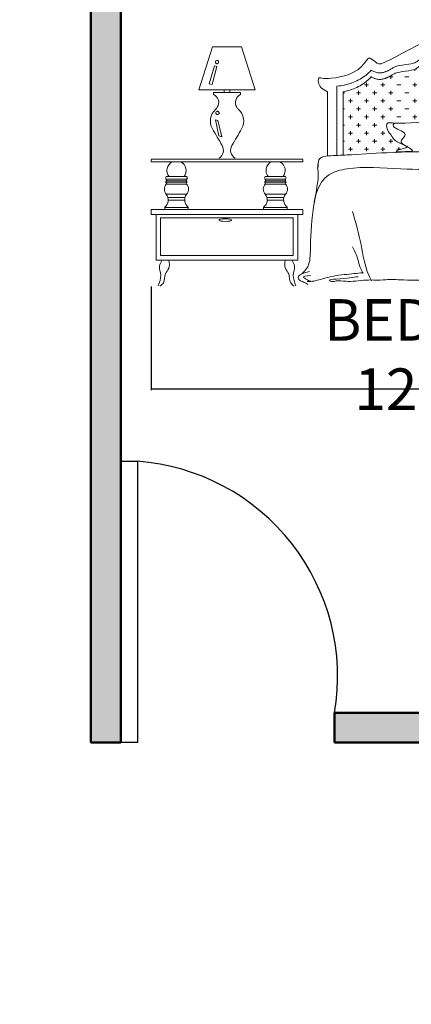
# Model space of a CAD drawing. Units: inches. Extents: x 1771 to 3025, y 319 to 889.
# Tile 20 of 35: x 2390 to 2456, y 621 to 786. Entities that reach past the tile are written whole.
import ezdxf

# ---------------------------------------------------------------- set-up
doc = ezdxf.new("R2010")
doc.units = ezdxf.units.IN
doc.header["$MEASUREMENT"] = 0
for name, color, linetype, lineweight in [('A-ANNO-DIMS', 2, 'Continuous', 18), ('A-AREA-IDEN', 241, 'Continuous', 25), ('A-DOOR', 4, 'Continuous', 25), ('A-FURN', 8, 'Continuous', 18), ('A-WALL', 7, 'Continuous', 50), ('A-WALL-PATT', 254, 'Continuous', 13)]:
    doc.layers.add(name, color=color, linetype=linetype, lineweight=lineweight)
doc.styles.get("Standard").update_dxf_attribs({"font": 'arial.ttf'})
doc.dimstyles.get("Standard").update_dxf_attribs({"dimtxt": 0.18, "dimasz": 0.18, "dimexe": 0.18, "dimexo": 0.0625, "dimgap": 0.09, "dimtad": 0, "dimtih": 1, "dimtoh": 1, "dimdec": 4, "dimzin": 0, "dimdsep": 46, "dimtxsty": 'Standard', "dimcen": 0.09, "dimadec": 0, "dimazin": 0, "dimtfac": 1, "dimtdec": 4, "dimtofl": 0, "dimtmove": 0, "dimatfit": 3, "dimfxl": 1, "dimtolj": 1, "dimtzin": 0, "dimarcsym": 0})

# ---------------------------------------------------------------- blocks, each defined once
blk = doc.blocks.new('A$C3F6F0378')
for p, q in [((188.6, 774.2), (242.7, 943.6)), ((356.2, 943.6), (242.7, 943.6)), ((410.4, 774.2), (356.2, 943.6)), ((1198.7, 944.7), (1198.7, 946.2)), ((1254.2, 952.6), (1270.1, 952.6)), ((1262.2, 944.7), (1262.2, 960.5)), ((1317.7, 952.6), (1333.6, 952.6)), ((1325.7, 944.7), (1325.7, 960.5)), ((1381.2, 952.6), (1397.1, 952.6)), ((1389.2, 944.7), (1389.2, 959.9)), ((2294.6, 774.2), (2348.7, 943.6)), ((2462.2, 943.6), (2348.7, 943.6)), ((2516.4, 774.2), (2462.2, 943.6)), ((1135.2, 881.2), (1135.2, 897)), ((1162.7, 920.9), (1174.9, 920.9)), ((1166.9, 912.9), (1166.9, 924)), ((1198.7, 881.2), (1198.7, 897)), ((1222.5, 920.9), (1238.4, 920.9)), ((1230.4, 912.9), (1230.4, 928.8)), ((1262.2, 881.2), (1262.2, 897)), ((1286, 920.9), (1301.9, 920.9)), ((1293.9, 912.9), (1293.9, 928.8)), ((1325.7, 881.2), (1325.7, 897)), ((1349.5, 920.9), (1365.4, 920.9)), ((1357.4, 912.9), (1357.4, 928.8)), ((1389.2, 881.2), (1389.2, 897)), ((1413, 920.9), (1428.9, 920.9)), ((1420.9, 912.9), (1420.9, 928.8)), ((1452.7, 881.2), (1452.7, 897)), ((1476.5, 920.9), (1485.8, 920.9)), ((1484.4, 912.9), (1484.4, 921.6)), ((1516.2, 881.2), (1516.2, 897)), ((1579.7, 881.2), (1579.7, 897)), ((229, 797.8), (250.3, 869.3)), ((259.4, 866.2), (241.2, 794.8)), ((250.3, 869.3), (259.4, 866.2)), ((1039.9, 849.4), (1039.9, 855.2)), ((1044.6, 857.4), (1047.9, 857.4)), ((1095.5, 857.4), (1111.4, 857.4)), ((1103.4, 849.4), (1103.4, 865.3)), ((1127.2, 889.1), (1143.1, 889.1)), ((1159, 857.4), (1174.9, 857.4)), ((1166.9, 849.4), (1166.9, 865.3)), ((1190.7, 889.1), (1206.6, 889.1)), ((1222.5, 857.4), (1238.4, 857.4)), ((1230.4, 849.4), (1230.4, 865.3)), ((1254.2, 889.1), (1270.1, 889.1)), ((1286, 857.4), (1301.9, 857.4)), ((1293.9, 849.4), (1293.9, 865.3)), ((1317.7, 889.1), (1333.6, 889.1)), ((1349.5, 857.4), (1365.4, 857.4)), ((1357.4, 849.4), (1357.4, 865.3)), ((1381.2, 889.1), (1397.1, 889.1)), ((1413, 857.4), (1428.9, 857.4)), ((1420.9, 849.4), (1420.9, 865.3)), ((1444.7, 889.1), (1460.6, 889.1)), ((1476.5, 857.4), (1492.4, 857.4)), ((1484.4, 849.4), (1484.4, 865.3)), ((1508.2, 889.1), (1524.1, 889.1)), ((1540, 857.4), (1555.9, 857.4)), ((1547.9, 849.4), (1547.9, 865.3)), ((1571.7, 889.1), (1587.6, 889.1)), ((1603.5, 857.4), (1619.4, 857.4)), ((1611.4, 849.4), (1611.4, 865.3)), ((2335.1, 797.8), (2356.3, 869.3)), ((2365.5, 866.2), (2347.3, 794.8)), ((2356.3, 869.3), (2365.5, 866.2)), ((881.2, 817.7), (881.2, 818.8)), ((937.5, 825.6), (952.6, 825.6)), ((944.7, 817.7), (944.7, 829.4)), ((1000.2, 825.6), (1016.1, 825.6)), ((1063.7, 825.6), (1079.6, 825.6)), ((1071.7, 817.7), (1071.7, 833.5)), ((1127.2, 825.6), (1143.1, 825.6)), ((1135.2, 817.7), (1135.2, 833.5)), ((1190.7, 825.6), (1206.6, 825.6)), ((1198.7, 817.7), (1198.7, 833.5)), ((1254.2, 825.6), (1270.1, 825.6)), ((1262.2, 817.7), (1262.2, 833.5)), ((1317.7, 825.6), (1333.6, 825.6)), ((1325.7, 817.7), (1325.7, 833.5)), ((1381.2, 825.6), (1397.1, 825.6)), ((1389.2, 817.7), (1389.2, 833.5)), ((1444.7, 825.6), (1460.6, 825.6)), ((1452.7, 817.7), (1452.7, 833.5)), ((1508.2, 825.6), (1524.1, 825.6)), ((1516.2, 817.7), (1516.2, 833.5)), ((1571.7, 825.6), (1587.6, 825.6)), ((1579.7, 817.7), (1579.7, 833.5)), ((1635.2, 825.6), (1651.1, 825.6)), ((1643.2, 817.7), (1643.2, 833.5)), ((1698.7, 825.6), (1714.6, 825.6)), ((1706.7, 817.7), (1706.7, 828.2)), ((1770.2, 818.9), (1770.2, 818.9)), ((241.2, 794.8), (229, 797.8)), ((841.5, 793.9), (857.4, 793.9)), ((849.4, 785.9), (849.4, 801.8)), ((905, 793.9), (920.9, 793.9)), ((912.9, 785.9), (912.9, 801.8)), ((968.5, 793.9), (984.4, 793.9)), ((1032, 793.9), (1047.9, 793.9)), ((1039.9, 785.9), (1039.9, 801.8)), ((1095.5, 793.9), (1111.4, 793.9)), ((1103.4, 785.9), (1103.4, 801.8)), ((1159, 793.9), (1174.9, 793.9)), ((1166.9, 785.9), (1166.9, 801.8)), ((1222.5, 793.9), (1238.4, 793.9)), ((1230.4, 785.9), (1230.4, 801.8)), ((1286, 793.9), (1301.9, 793.9)), ((1293.9, 785.9), (1293.9, 801.8)), ((1349.5, 793.9), (1365.4, 793.9)), ((1357.4, 785.9), (1357.4, 801.8)), ((1413, 793.9), (1428.9, 793.9)), ((1420.9, 785.9), (1420.9, 801.8)), ((1476.5, 793.9), (1492.4, 793.9)), ((1484.4, 785.9), (1484.4, 801.8)), ((1540, 793.9), (1555.9, 793.9)), ((1547.9, 785.9), (1547.9, 801.8)), ((1603.5, 793.9), (1619.4, 793.9)), ((1611.4, 785.9), (1611.4, 801.8)), ((1667, 793.9), (1682.9, 793.9)), ((1674.9, 785.9), (1674.9, 801.8)), ((1730.5, 793.9), (1746.4, 793.9)), ((1738.4, 785.9), (1738.4, 801.8)), ((1794, 793.9), (1809.9, 793.9)), ((1801.9, 785.9), (1801.9, 801.8)), ((1857.5, 793.9), (1863, 793.9)), ((1865.4, 785.9), (1865.4, 792.4)), ((2347.3, 794.8), (2335.1, 797.8)), ((410.4, 774.2), (188.6, 774.2)), ((246.2, 763), (246.2, 755.2)), ((246.2, 763), (246.2, 755.2)), ((352.5, 763), (246.2, 763)), ((287.7, 774.2), (287.7, 763)), ((311, 763), (287.7, 763)), ((311, 774.2), (311, 763)), ((352.5, 763), (352.5, 755.2)), ((352.5, 763), (352.5, 755.2)), ((757.1, 762.1), (762.1, 762.1)), ((785.9, 722.4), (785.9, 738.3)), ((809.7, 762.1), (825.6, 762.1)), ((817.7, 754.2), (817.7, 770)), ((849.4, 722.4), (849.4, 738.3)), ((873.2, 762.1), (889.1, 762.1)), ((881.2, 754.2), (881.2, 770)), ((912.9, 722.4), (912.9, 738.3)), ((936.7, 762.1), (952.6, 762.1)), ((944.7, 754.2), (944.7, 770)), ((1000.2, 762.1), (1016.1, 762.1)), ((1039.9, 722.4), (1039.9, 738.3)), ((1063.7, 762.1), (1079.6, 762.1)), ((1071.7, 754.2), (1071.7, 770)), ((1103.4, 722.4), (1103.4, 738.3)), ((1127.2, 762.1), (1143.1, 762.1)), ((1135.2, 754.2), (1135.2, 770)), ((1166.9, 722.4), (1166.9, 738.3)), ((1190.7, 762.1), (1206.6, 762.1)), ((1198.7, 754.2), (1198.7, 770)), ((1230.4, 722.4), (1230.4, 738.3)), ((1254.2, 762.1), (1270.1, 762.1)), ((1262.2, 754.2), (1262.2, 770)), ((1293.9, 722.4), (1293.9, 738.3)), ((1317.7, 762.1), (1333.6, 762.1)), ((1325.7, 754.2), (1325.7, 770)), ((1357.4, 722.4), (1357.4, 738.3)), ((1381.2, 762.1), (1397.1, 762.1)), ((1389.2, 754.2), (1389.2, 770)), ((1420.9, 722.4), (1420.9, 738.3)), ((1444.7, 762.1), (1460.6, 762.1)), ((1452.7, 754.2), (1452.7, 770)), ((1484.4, 722.4), (1484.4, 738.3)), ((1508.2, 762.1), (1524.1, 762.1)), ((1516.2, 754.2), (1516.2, 770)), ((1547.9, 723.4), (1547.9, 738.3)), ((1571.7, 762.1), (1587.6, 762.1)), ((1579.7, 754.2), (1579.7, 770)), ((1611.4, 732.6), (1611.4, 738.3)), ((1635.2, 762.1), (1651.1, 762.1)), ((1643.2, 754.2), (1643.2, 770)), ((1698.7, 762.1), (1714.6, 762.1)), ((1706.7, 754.2), (1706.7, 770)), ((1762.2, 762.1), (1778.1, 762.1)), ((1801.9, 722.4), (1801.9, 738.3)), ((1825.7, 762.1), (1841.6, 762.1)), ((1833.7, 754.2), (1833.7, 770)), ((1865.4, 722.4), (1865.4, 738.3)), ((1889.2, 762.1), (1905.1, 762.1)), ((1897.2, 754.2), (1897.2, 770)), ((1928.9, 722.4), (1928.9, 738.3)), ((2516.4, 774.2), (2294.6, 774.2)), ((2352.3, 763), (2352.3, 755.2)), ((2352.3, 763), (2352.3, 755.2)), ((2458.6, 763), (2352.3, 763)), ((2393.8, 774.2), (2393.8, 763)), ((2417.1, 763), (2393.8, 763)), ((2417.1, 774.2), (2417.1, 763)), ((2458.6, 763), (2458.6, 755.2)), ((2458.6, 763), (2458.6, 755.2)), ((778, 730.4), (793.9, 730.4)), ((817.7, 690.7), (817.7, 706.5)), ((841.5, 730.4), (857.4, 730.4)), ((881.2, 690.7), (881.2, 706.5)), ((905, 730.4), (920.9, 730.4)), ((944.7, 690.7), (944.7, 706.5)), ((968.5, 730.4), (984.4, 730.4)), ((1032, 730.4), (1047.9, 730.4)), ((1071.7, 690.7), (1071.7, 706.5)), ((1095.5, 730.4), (1111.4, 730.4)), ((1135.2, 690.7), (1135.2, 706.5)), ((1159, 730.4), (1174.9, 730.4)), ((1198.7, 690.7), (1198.7, 706.5)), ((1222.5, 730.4), (1238.4, 730.4)), ((1286, 730.4), (1301.9, 730.4)), ((1349.5, 730.4), (1365.4, 730.4)), ((1413, 730.4), (1428.9, 730.4)), ((1476.5, 730.4), (1492.4, 730.4)), ((1540, 730.4), (1555.9, 730.4)), ((1770.2, 690.7), (1770.2, 706.5)), ((1794, 730.4), (1809.9, 730.4)), ((1833.7, 690.7), (1833.7, 706.5)), ((1857.5, 730.4), (1873.4, 730.4)), ((1897.2, 690.7), (1897.2, 706.5)), ((1921, 730.4), (1935.3, 730.4)), ((757.1, 698.6), (762.1, 698.6)), ((778, 666.9), (793.9, 666.9)), ((785.9, 658.9), (785.9, 674.8)), ((809.7, 698.6), (825.6, 698.6)), ((841.5, 666.9), (857.4, 666.9)), ((849.4, 658.9), (849.4, 674.8)), ((873.2, 698.6), (889.1, 698.6)), ((905, 666.9), (920.9, 666.9)), ((912.9, 658.9), (912.9, 674.8)), ((936.7, 698.6), (952.6, 698.6)), ((968.5, 666.9), (984.4, 666.9)), ((1000.2, 698.6), (1016.1, 698.6)), ((1032, 666.9), (1047.9, 666.9)), ((1039.9, 658.9), (1039.9, 674.8)), ((1063.7, 698.6), (1079.6, 698.6)), ((1095.5, 666.9), (1111.4, 666.9)), ((1103.4, 658.9), (1103.4, 674.8)), ((1127.2, 698.6), (1143.1, 698.6)), ((1159, 666.9), (1174.9, 666.9)), ((1166.9, 658.9), (1166.9, 674.8)), ((1190.7, 698.6), (1206.6, 698.6)), ((1222.5, 666.9), (1238.4, 666.9)), ((1230.4, 658.9), (1230.4, 674.8)), ((1765.2, 698.6), (1778.1, 698.6)), ((1794, 666.9), (1809.9, 666.9)), ((1801.9, 658.9), (1801.9, 674.8)), ((1825.7, 698.6), (1841.6, 698.6)), ((1857.5, 666.9), (1873.4, 666.9)), ((1865.4, 658.9), (1865.4, 674.8)), ((1889.2, 698.6), (1905.1, 698.6)), ((1921, 666.9), (1935.3, 666.9)), ((1928.9, 658.9), (1928.9, 674.8)), ((253.5, 655.6), (262.6, 652.5)), ((267.2, 592.3), (253.5, 655.6)), ((262.6, 652.5), (279.4, 589.2)), ((757.1, 635.1), (762.1, 635.1)), ((809.7, 635.1), (825.6, 635.1)), ((817.7, 627.2), (817.7, 643)), ((873.2, 635.1), (889.1, 635.1)), ((881.2, 627.2), (881.2, 643)), ((1764.2, 635.1), (1778.1, 635.1)), ((1770.2, 627.2), (1770.2, 643)), ((1825.7, 635.1), (1841.6, 635.1)), ((1833.7, 627.2), (1833.7, 643)), ((1889.2, 635.1), (1905.1, 635.1)), ((1897.2, 627.2), (1897.2, 643)), ((2359.5, 655.6), (2368.6, 652.5)), ((2373.2, 592.3), (2359.5, 655.6)), ((2368.6, 652.5), (2385.4, 589.2)), ((279.4, 589.2), (267.2, 592.3)), ((778, 603.4), (793.9, 603.4)), ((785.9, 595.4), (785.9, 611.3)), ((841.5, 603.4), (857.4, 603.4)), ((849.4, 595.4), (849.4, 611.3)), ((905, 603.4), (920.9, 603.4)), ((912.9, 595.4), (912.9, 611.3)), ((1794, 603.4), (1809.9, 603.4)), ((1801.9, 595.4), (1801.9, 611.3)), ((1857.5, 603.4), (1873.4, 603.4)), ((1865.4, 595.4), (1865.4, 611.3)), ((1921, 603.4), (1935.3, 603.4)), ((1928.9, 595.4), (1928.9, 611.3)), ((2385.4, 589.2), (2373.2, 592.3)), ((757.1, 571.6), (762.1, 571.6)), ((785.9, 531.9), (785.9, 547.8)), ((809.7, 571.6), (825.6, 571.6)), ((817.7, 563.7), (817.7, 579.5)), ((849.4, 531.9), (849.4, 547.8)), ((873.2, 571.6), (889.1, 571.6)), ((881.2, 563.7), (881.2, 579.5)), ((912.9, 531.9), (912.9, 547.8)), ((936.7, 571.6), (952.6, 571.6)), ((944.7, 563.7), (944.7, 579.5)), ((976.4, 536.8), (976.4, 547.8)), ((1764.5, 571.6), (1778.1, 571.6)), ((1770.2, 563.7), (1770.2, 579.5)), ((1801.9, 531.9), (1801.9, 547.8)), ((1825.7, 571.6), (1841.6, 571.6)), ((1833.7, 563.7), (1833.7, 579.5)), ((1865.4, 531.9), (1865.4, 547.8)), ((1889.2, 571.6), (1905.1, 571.6)), ((1897.2, 563.7), (1897.2, 579.5)), ((1928.9, 531.9), (1928.9, 547.8)), ((778, 539.9), (793.9, 539.9)), ((841.5, 539.9), (857.4, 539.9)), ((905, 539.9), (920.9, 539.9)), ((968.5, 539.9), (984.4, 539.9)), ((1794, 539.9), (1809.9, 539.9)), ((1857.5, 539.9), (1873.4, 539.9)), ((1921, 539.9), (1935.3, 539.9)), ((598.4, 500), (0, 500)), ((0, 499.7), (0, 489.7)), ((598.4, 490), (0, 490)), ((598.4, 499.7), (598.4, 489.7)), ((658.9, 468.4), (658.9, 484.3)), ((2704.5, 500), (2106.1, 500)), ((2106.1, 499.7), (2106.1, 489.7)), ((2704.5, 490), (2106.1, 490)), ((2704.5, 499.7), (2704.5, 489.7)), ((140, 432.2), (60, 432.2)), ((140, 432.2), (60, 432.2)), ((529.9, 432.2), (449.9, 432.2)), ((529.9, 432.2), (449.9, 432.2)), ((2246.1, 432.2), (2166.1, 432.2)), ((2246.1, 432.2), (2166.1, 432.2)), ((2635.9, 432.2), (2555.9, 432.2)), ((2635.9, 432.2), (2555.9, 432.2)), ((141.9, 409.3), (58.1, 409.3)), ((140, 422.2), (60, 422.2)), ((140, 402.2), (60, 402.2)), ((138.2, 415.4), (61.8, 415.4)), ((531.8, 409.3), (447.9, 409.3)), ((529.9, 422.2), (449.9, 422.2)), ((529.9, 402.2), (449.9, 402.2)), ((528.1, 415.4), (451.7, 415.4)), ((2248, 409.3), (2164.1, 409.3)), ((2246.1, 422.2), (2166.1, 422.2)), ((2246.1, 402.2), (2166.1, 402.2)), ((2244.2, 415.4), (2167.9, 415.4)), ((2637.9, 409.3), (2554, 409.3)), ((2635.9, 422.2), (2555.9, 422.2)), ((2635.9, 402.2), (2555.9, 402.2)), ((2634.1, 415.4), (2557.7, 415.4)), ((140, 362.2), (60, 362.2)), ((529.9, 362.2), (449.9, 362.2)), ((2246.1, 362.2), (2166.1, 362.2)), ((2635.9, 362.2), (2555.9, 362.2)), ((53.7, 311), (53.7, 302.2)), ((133.7, 349.2), (66.3, 349.2)), ((132.4, 338.7), (67.5, 338.7)), ((146.3, 311), (146.3, 302.2)), ((443.6, 311), (443.6, 302.2)), ((523.5, 349.2), (456.2, 349.2)), ((522.3, 338.7), (457.4, 338.7)), ((536.1, 311), (536.1, 302.2)), ((2159.8, 311), (2159.8, 302.2)), ((2239.7, 349.2), (2172.4, 349.2)), ((2238.5, 338.7), (2173.6, 338.7)), ((2252.3, 311), (2252.3, 302.2)), ((2549.7, 311), (2549.7, 302.2)), ((2629.6, 349.2), (2562.2, 349.2)), ((2628.4, 338.7), (2563.5, 338.7)), ((2642.2, 311), (2642.2, 302.2)), ((0, 302.2), (0, 282.2)), ((598.4, 302.2), (0, 302.2)), ((598.4, 282.2), (0, 282.2)), ((20, 282.2), (20, 102.2)), ((146.3, 310.3), (53.7, 310.3)), ((80, 302.2), (120, 302.2)), ((80, 302.2), (130, 302.2)), ((536.1, 310.3), (443.6, 310.3)), ((469.9, 302.2), (509.9, 302.2)), ((469.9, 302.2), (519.9, 302.2)), ((578.4, 102.2), (578.4, 282.2)), ((598.4, 282.2), (598.4, 302.2)), ((2106.1, 302.2), (2106.1, 282.2)), ((2704.5, 302.2), (2106.1, 302.2)), ((2704.5, 282.2), (2106.1, 282.2)), ((2126.1, 282.2), (2126.1, 102.2)), ((2252.3, 310.3), (2159.8, 310.3)), ((2186.1, 302.2), (2226.1, 302.2)), ((2186.1, 302.2), (2236.1, 302.2)), ((2642.2, 310.3), (2549.7, 310.3)), ((2575.9, 302.2), (2615.9, 302.2)), ((2575.9, 302.2), (2625.9, 302.2)), ((2684.5, 102.2), (2684.5, 282.2)), ((2704.5, 282.2), (2704.5, 302.2)), ((37.2, 268.9), (560.2, 268.9)), ((37.2, 120.8), (37.2, 268.9)), ((560.2, 268.9), (560.2, 120.8)), ((2143.3, 268.9), (2666.3, 268.9)), ((2143.3, 120.8), (2143.3, 268.9)), ((2666.3, 268.9), (2666.3, 120.8)), ((560.2, 120.8), (37.2, 120.8)), ((2666.3, 120.8), (2143.3, 120.8)), ((20, 102.2), (578.4, 102.2)), ((2126.1, 102.2), (2684.5, 102.2))]:
    blk.add_line(p, q)
at = {"ltscale": 20}
for p, q in [((732.5, 788.3), (732.5, 515.5)), ((1959.8, 788.3), (1959.8, 515.7)), ((695.7, 766.2), (695.7, 513.2)), ((757.1, 766), (757.1, 516.6)), ((1935.3, 766), (1935.3, 516.7)), ((1996.6, 766.2), (1996.6, 513.5))]:
    blk.add_line(p, q, dxfattribs=at)
for centre in [(1320.3, 981.3), (1320.4, 945.7), (1320.4, 919.9)]:
    blk.add_arc(centre, 55.2, 80.5605, 99.4395, dxfattribs=at)
for centre, radius, start, end in [((259.7, 883.6), 6.48, 168.6084, 233.2112), ((259.7, 883.6), 6.49, 104.0344, 168.6084), ((259.6, 883.5), 6.42, 233.2112, 255.9722), ((260, 883.6), 6.51, 78.6968, 107.1924), ((259.7, 883.8), 6.69, 255.9722, 278.2688), ((259.7, 883.9), 6.81, 278.2688, 342.9026), ((260, 883.7), 6.5, 50.1648, 78.6968), ((260.1, 883.8), 6.35, 342.9026, 50.1648), ((2365.7, 883.6), 6.48, 168.6084, 233.2112), ((2365.7, 883.6), 6.49, 104.0344, 168.6084), ((2365.7, 883.5), 6.42, 233.2112, 255.9722), ((2366.1, 883.6), 6.51, 78.6968, 107.1924), ((2365.7, 883.8), 6.69, 255.9722, 278.2688), ((2365.7, 883.9), 6.81, 278.2688, 342.9026), ((2366.1, 883.7), 6.5, 50.1648, 78.6968), ((2366.2, 883.8), 6.35, 342.9026, 50.1648), ((232.6, 724.1), 33.9, 326.6744, 66.3416), ((366.1, 724.1), 33.9, 113.6584, 213.3256), ((2338.7, 724.1), 33.9, 326.6744, 66.3416), ((2472.2, 724.1), 33.9, 113.6584, 213.3256), ((231, 722.3), 34.4, 312.0366, 330.6067), ((367.7, 722.3), 34.4, 209.3933, 227.9634), ((2337, 722.3), 34.4, 312.0366, 330.6067), ((2473.8, 722.3), 34.4, 209.3933, 227.9634), ((295.2, 651.2), 61.5, 132.0366, 209.8723), ((261.7, 682.8), 6.48, 168.6084, 233.2112), ((261.7, 682.8), 6.49, 104.0344, 168.6084), ((261.6, 682.8), 6.42, 233.2112, 255.9722), ((262, 682.9), 6.51, 78.6968, 107.1924), ((261.7, 683), 6.69, 255.9722, 278.2688), ((261.7, 683.1), 6.81, 278.2688, 342.9026), ((262, 682.9), 6.5, 50.1648, 78.6968), ((262.1, 683), 6.35, 342.9026, 50.1648), ((303.6, 651.2), 61.5, 330.1277, 47.9634), ((2401.2, 651.2), 61.5, 132.0366, 209.8723), ((2367.7, 682.8), 6.48, 168.6084, 233.2112), ((2367.7, 682.8), 6.49, 104.0344, 168.6084), ((2367.7, 682.8), 6.42, 233.2112, 255.9722), ((2367.8, 683), 6.69, 255.9722, 278.2688), ((2368.1, 682.9), 6.51, 78.6968, 107.1924), ((2367.8, 683.1), 6.81, 278.2688, 342.9026), ((2368.1, 682.9), 6.5, 50.1648, 78.6968), ((2368.2, 683), 6.35, 342.9026, 50.1648), ((2409.6, 651.2), 61.5, 330.1277, 47.9634), ((9112.8, 5715.8), 10230.1, 209.87228, 210.29853), ((-8514, 5715.8), 10230.1, 329.70147, 330.12772), ((11218.8, 5715.8), 10230.1, 209.87228, 210.29853), ((-6408, 5715.8), 10230.1, 329.70147, 330.12772), ((247.8, 535.9), 37.3, 302.5427, 30.2985), ((350.9, 535.9), 37.3, 149.7015, 237.4573), ((2353.9, 535.9), 37.3, 302.5427, 30.2985), ((2457, 535.9), 37.3, 149.7015, 237.4573), ((100.5, 456.1), 37.8, 115.9414, 219.2084), ((100.5, 456.1), 37.8, 320.7916, 64.0586), ((490.9, 456.1), 37.8, 115.9414, 219.2084), ((490.9, 456.1), 37.8, 320.7916, 64.0586), ((2206.6, 456.1), 37.8, 115.9414, 219.2084), ((2206.6, 456.1), 37.8, 320.7916, 64.0586), ((2597, 456.1), 37.8, 115.9414, 219.2084), ((2597, 456.1), 37.8, 320.7916, 64.0586), ((63.7, 427.2), 6.24, 126.78, 233.22), ((136.2, 427.2), 6.24, 306.78, 53.22), ((453.6, 427.2), 6.24, 126.78, 233.22), ((526.1, 427.2), 6.24, 306.78, 53.22), ((2169.8, 427.2), 6.24, 126.78, 233.22), ((2242.3, 427.2), 6.24, 306.78, 53.22), ((2559.7, 427.2), 6.24, 126.78, 233.22), ((2632.2, 427.2), 6.24, 306.78, 53.22), ((82, 382.2), 29.7, 137.7452, 222.2548), ((118, 382.2), 29.7, 317.7452, 42.2548), ((471.9, 382.2), 29.7, 137.7452, 222.2548), ((507.8, 382.2), 29.7, 317.7452, 42.2548), ((2188.1, 382.2), 29.7, 137.7452, 222.2548), ((2224, 382.2), 29.7, 317.7452, 42.2548), ((2577.9, 382.2), 29.7, 137.7452, 222.2548), ((2613.9, 382.2), 29.7, 317.7452, 42.2548), ((30.6, 339.8), 37, 308.7547, 37.2668), ((169.4, 339.8), 37, 142.7332, 231.2453), ((420.5, 339.8), 37, 308.7547, 37.2668), ((559.3, 339.8), 37, 142.7332, 231.2453), ((2136.7, 339.8), 37, 308.7547, 37.2668), ((2275.4, 339.8), 37, 142.7332, 231.2453), ((2526.5, 339.8), 37, 308.7547, 37.2668), ((2665.3, 339.8), 37, 142.7332, 231.2453)]:
    blk.add_arc(centre, radius, start, end)
for centre in [(292.3, 260.1), (2398.3, 260.1)]:
    blk.add_ellipse(centre, major_axis=(25, 0), ratio=0.2)
for points, knots in [([(695.7, 766.2), (675.2, 775.8), (657.2, 791.6), (658.6, 824.3), (675.7, 817.9), (731.9, 819.9), (817.7, 836.7), (863.4, 913.8), (889.3, 869.9), (957.4, 896.6), (1128.9, 1003.6), (1245.7, 1025), (1311.4, 1035.8)], [12.417853, 12.417853, 12.417853, 12.417853, 68.394536, 90.665986, 114.156853, 157.554067, 281.869614, 298.858744, 338.737111, 347.060176, 470.423438, 625.498764, 625.498764, 625.498764, 625.498764]), ([(1996.6, 766.2), (2017.1, 775.8), (2035.1, 791.6), (2033.8, 824.3), (2016.6, 817.9), (1960.4, 819.9), (1874.7, 836.7), (1829, 913.8), (1803, 869.9), (1652.5, 896.6), (1584, 1003.6), (1395.1, 1025), (1329.4, 1035.8)], [12.417853, 12.417853, 12.417853, 12.417853, 68.394536, 90.665986, 114.156853, 157.554067, 281.869614, 298.858744, 338.737111, 347.060176, 470.423438, 625.498764, 625.498764, 625.498764, 625.498764]), ([(867.4, 851.3), (868.1, 850.9), (868.9, 850.4), (871.2, 849.1), (872.9, 848.2), (876.8, 846.3), (879, 845.4), (884, 843.6), (886.7, 842.8), (892, 841.7), (894.6, 841.4), (898.4, 841.1), (899.4, 841), (901.2, 841), (901.9, 841), (903.1, 841), (903.7, 841.1), (904.8, 841.1), (905.4, 841.2), (907, 841.3), (908.1, 841.4), (911.6, 841.9), (913.8, 842.3), (917.8, 843.3), (919.6, 843.9), (922.7, 844.9), (924.1, 845.5), (926.6, 846.4), (927.6, 846.9), (928.8, 847.4), (929.1, 847.5), (929.7, 847.8), (929.9, 847.9), (930.7, 848.2), (931.3, 848.5), (932.9, 849.2), (933.9, 849.7), (937.1, 851.3), (939.2, 852.3), (945.3, 855.5), (949.2, 857.8), (959.8, 864.4), (966.2, 869), (1040, 878.3), (1045.6, 883.1), (1056.3, 892.7), (1061.3, 897.5), (1112.2, 907), (1116.8, 911.6), (1125.6, 920.6), (1129.9, 924.9), (1138.3, 933), (1142.3, 936.8), (1148.2, 942), (1150, 943.5), (1153.3, 946.3), (1154.7, 947.4), (1157, 949.2), (1157.9, 949.9), (1159.7, 951.2), (1160.6, 951.8), (1163.4, 953.8), (1165.3, 955), (1171, 958.7), (1174.9, 961), (1186, 967), (1193.5, 970.4), (1209.3, 976.7), (1217.6, 979.5), (1235, 984.7), (1244, 987), (1262.7, 991.3), (1272.4, 993.3), (1291.8, 996.9), (1301.5, 998.6), (1311.3, 1000.2)], [328.6705, 328.6705, 328.6705, 328.6705, 329.609368, 329.609368, 331.487103, 331.487103, 333.620342, 333.620342, 335.753581, 335.753581, 337.507866, 337.507866, 338.182373, 338.182373, 338.607397, 338.607397, 338.959312, 338.959312, 339.311227, 339.311227, 340.015058, 340.015058, 341.722742, 341.722742, 343.430427, 343.430427, 345.138111, 345.138111, 346.845796, 346.845796, 347.37881, 347.37881, 347.911824, 347.911824, 348.977853, 348.977853, 351.109909, 351.109909, 355.374023, 355.374023, 363.902249, 363.902249, 379.258481, 379.258481, 394.614712, 394.614712, 409.970944, 409.970944, 425.327175, 425.327175, 440.683406, 440.683406, 456.039638, 456.039638, 463.285514, 463.285514, 469.01116, 469.01116, 472.593, 472.593, 476.17484, 476.17484, 483.338521, 483.338521, 497.665882, 497.665882, 522.309302, 522.309302, 546.952723, 546.952723, 571.596143, 571.596143, 596.239564, 596.239564, 619.876409, 619.876409, 619.876409, 619.876409]), ([(867.4, 825.4), (868.1, 825), (868.9, 824.6), (871.2, 823.2), (872.9, 822.3), (876.8, 820.5), (879, 819.5), (884, 817.8), (886.7, 817), (892, 815.9), (894.6, 815.5), (898.4, 815.2), (899.4, 815.2), (901.2, 815.2), (901.9, 815.2), (903.1, 815.2), (903.7, 815.2), (904.8, 815.3), (905.4, 815.3), (907, 815.4), (908.1, 815.5), (911.6, 816), (913.8, 816.5), (917.8, 817.5), (919.6, 818), (922.7, 819.1), (924.1, 819.6), (926.6, 820.6), (927.6, 821), (928.8, 821.5), (929.1, 821.7), (929.7, 821.9), (929.9, 822), (930.7, 822.4), (931.3, 822.6), (932.9, 823.4), (933.9, 823.9), (937.1, 825.4), (939.2, 826.4), (945.3, 829.7), (949.2, 832), (959.8, 838.6), (966.2, 843.1), (1040, 852.4), (1045.6, 857.2), (1056.3, 866.8), (1061.3, 871.6), (1112.2, 881.1), (1116.8, 885.7), (1125.6, 894.7), (1129.9, 899), (1138.3, 907.1), (1142.3, 910.9), (1148.2, 916.1), (1150, 917.7), (1153.3, 920.4), (1154.7, 921.5), (1157, 923.3), (1157.9, 924), (1159.7, 925.3), (1160.6, 926), (1163.4, 927.9), (1165.3, 929.2), (1171, 932.8), (1174.9, 935.2), (1186, 941.1), (1193.5, 944.6), (1209.3, 950.8), (1217.6, 953.7), (1235, 958.8), (1244, 961.2), (1262.7, 965.5), (1272.4, 967.4), (1291.8, 971), (1301.5, 972.7), (1311.3, 974.3)], [328.6705, 328.6705, 328.6705, 328.6705, 329.609368, 329.609368, 331.487103, 331.487103, 333.620342, 333.620342, 335.753581, 335.753581, 337.507866, 337.507866, 338.182373, 338.182373, 338.607397, 338.607397, 338.959312, 338.959312, 339.311227, 339.311227, 340.015058, 340.015058, 341.722742, 341.722742, 343.430427, 343.430427, 345.138111, 345.138111, 346.845796, 346.845796, 347.37881, 347.37881, 347.911824, 347.911824, 348.977853, 348.977853, 351.109909, 351.109909, 355.374023, 355.374023, 363.902249, 363.902249, 379.258481, 379.258481, 394.614712, 394.614712, 409.970944, 409.970944, 425.327175, 425.327175, 440.683406, 440.683406, 456.039638, 456.039638, 463.285514, 463.285514, 469.01116, 469.01116, 472.593, 472.593, 476.17484, 476.17484, 483.338521, 483.338521, 497.665882, 497.665882, 522.309302, 522.309302, 546.952723, 546.952723, 571.596143, 571.596143, 596.239564, 596.239564, 619.876409, 619.876409, 619.876409, 619.876409]), ([(1824.9, 851.3), (1824.2, 850.9), (1823.5, 850.4), (1821.1, 849.1), (1819.5, 848.2), (1815.6, 846.3), (1813.3, 845.4), (1808.4, 843.6), (1805.7, 842.8), (1800.3, 841.7), (1797.7, 841.4), (1794, 841.1), (1792.9, 841), (1791.2, 841), (1790.5, 841), (1789.2, 841), (1788.6, 841.1), (1787.5, 841.1), (1787, 841.2), (1785.3, 841.3), (1784.3, 841.4), (1780.8, 841.9), (1778.6, 842.3), (1774.6, 843.3), (1772.8, 843.9), (1769.6, 844.9), (1768.2, 845.5), (1765.8, 846.4), (1764.7, 846.9), (1763.5, 847.4), (1763.2, 847.5), (1762.7, 847.8), (1762.4, 847.9), (1761.6, 848.2), (1761.1, 848.5), (1759.5, 849.2), (1758.4, 849.7), (1755.2, 851.3), (1753.2, 852.3), (1664.6, 855.5), (1660.7, 857.8), (1650.1, 864.4), (1643.7, 869), (1631.7, 878.3), (1626.1, 883.1), (1615.5, 892.7), (1610.4, 897.5), (1600.8, 907), (1596.2, 911.6), (1587.3, 920.6), (1583, 924.9), (1574.7, 933), (1570.6, 936.8), (1492.6, 942), (1490.8, 943.5), (1487.5, 946.3), (1486.1, 947.4), (1483.8, 949.2), (1482.9, 949.9), (1481.1, 951.2), (1480.2, 951.8), (1477.4, 953.8), (1475.5, 955), (1469.8, 958.7), (1465.9, 961), (1454.8, 967), (1447.3, 970.4), (1431.5, 976.7), (1423.2, 979.5), (1405.8, 984.7), (1396.8, 987), (1378.1, 991.3), (1368.4, 993.3), (1349, 996.9), (1339.3, 998.6), (1329.5, 1000.2)], [328.6705, 328.6705, 328.6705, 328.6705, 329.609368, 329.609368, 331.487103, 331.487103, 333.620342, 333.620342, 335.753581, 335.753581, 337.507866, 337.507866, 338.182373, 338.182373, 338.607397, 338.607397, 338.959312, 338.959312, 339.311227, 339.311227, 340.015058, 340.015058, 341.722742, 341.722742, 343.430427, 343.430427, 345.138111, 345.138111, 346.845796, 346.845796, 347.37881, 347.37881, 347.911824, 347.911824, 348.977853, 348.977853, 351.109909, 351.109909, 355.374023, 355.374023, 363.902249, 363.902249, 379.258481, 379.258481, 394.614712, 394.614712, 409.970943, 409.970943, 425.327175, 425.327175, 440.683406, 440.683406, 456.039637, 456.039637, 463.285514, 463.285514, 469.011154, 469.011154, 472.592992, 472.592992, 476.17483, 476.17483, 483.338506, 483.338506, 497.665857, 497.665857, 522.309275, 522.309275, 546.952693, 546.952693, 571.59611, 571.59611, 596.239528, 596.239528, 619.876409, 619.876409, 619.876409, 619.876409]), ([(1824.9, 825.4), (1824.2, 825), (1823.5, 824.6), (1821.1, 823.2), (1819.5, 822.3), (1815.6, 820.5), (1813.3, 819.5), (1808.4, 817.8), (1805.7, 817), (1800.3, 815.9), (1797.7, 815.5), (1794, 815.2), (1792.9, 815.2), (1791.2, 815.2), (1790.5, 815.2), (1789.2, 815.2), (1788.6, 815.2), (1787.5, 815.3), (1787, 815.3), (1785.3, 815.4), (1784.3, 815.5), (1780.8, 816), (1778.6, 816.5), (1774.6, 817.5), (1772.8, 818), (1769.6, 819.1), (1768.2, 819.6), (1765.8, 820.6), (1764.7, 821), (1763.5, 821.5), (1763.2, 821.7), (1762.7, 821.9), (1762.4, 822), (1761.6, 822.4), (1761.1, 822.6), (1759.5, 823.4), (1758.4, 823.9), (1755.2, 825.4), (1753.2, 826.4), (1664.6, 829.7), (1660.7, 832), (1650.1, 838.6), (1643.7, 843.1), (1631.7, 852.4), (1626.1, 857.2), (1615.5, 866.8), (1610.4, 871.6), (1600.8, 881.1), (1596.2, 885.7), (1587.3, 894.7), (1583, 899), (1574.7, 907.1), (1570.6, 910.9), (1492.6, 916.1), (1490.8, 917.7), (1487.5, 920.4), (1486.1, 921.5), (1483.8, 923.3), (1482.9, 924), (1481.1, 925.3), (1480.2, 926), (1477.4, 927.9), (1475.5, 929.2), (1469.8, 932.8), (1465.9, 935.2), (1454.8, 941.1), (1447.3, 944.6), (1431.5, 950.8), (1423.2, 953.7), (1405.8, 958.8), (1396.8, 961.2), (1378.1, 965.5), (1368.4, 967.4), (1349, 971), (1339.3, 972.7), (1329.5, 974.3)], [328.6705, 328.6705, 328.6705, 328.6705, 329.609368, 329.609368, 331.487103, 331.487103, 333.620342, 333.620342, 335.753581, 335.753581, 337.507866, 337.507866, 338.182373, 338.182373, 338.607397, 338.607397, 338.959312, 338.959312, 339.311227, 339.311227, 340.015058, 340.015058, 341.722742, 341.722742, 343.430427, 343.430427, 345.138111, 345.138111, 346.845796, 346.845796, 347.37881, 347.37881, 347.911824, 347.911824, 348.977853, 348.977853, 351.109909, 351.109909, 355.374023, 355.374023, 363.902249, 363.902249, 379.258481, 379.258481, 394.614712, 394.614712, 409.970943, 409.970943, 425.327175, 425.327175, 440.683406, 440.683406, 456.039637, 456.039637, 463.285514, 463.285514, 469.011154, 469.011154, 472.592992, 472.592992, 476.17483, 476.17483, 483.338506, 483.338506, 497.665857, 497.665857, 522.309275, 522.309275, 546.952693, 546.952693, 571.59611, 571.59611, 596.239528, 596.239528, 619.876409, 619.876409, 619.876409, 619.876409]), ([(732.5, 788.3), (744.7, 789.4), (752.5, 790.8), (768.6, 794.5), (777, 796.7), (793.9, 802.3), (802.4, 805.7), (819.3, 813.7), (827.7, 818.4), (842.6, 828.5), (849.2, 833.6), (859.6, 843.1), (863.6, 847.1), (867.4, 851.3)], [179.330708, 179.330708, 179.330708, 179.330708, 196.086144, 196.086144, 213.445516, 213.445516, 230.804888, 230.804888, 248.16426, 248.16426, 262.451931, 262.451931, 271.832526, 271.832526, 271.832526, 271.832526]), ([(757.1, 766), (758.2, 766.3), (759.3, 766.5), (768.6, 768.6), (777, 770.9), (793.9, 776.5), (802.4, 779.8), (819.3, 787.9), (827.7, 792.6), (842.6, 802.7), (849.2, 807.8), (859.6, 817.2), (863.6, 821.2), (867.4, 825.4)], [193.740688, 193.740688, 193.740688, 193.740688, 196.086144, 196.086144, 213.445516, 213.445516, 230.804888, 230.804888, 248.16426, 248.16426, 262.451931, 262.451931, 271.832526, 271.832526, 271.832526, 271.832526]), ([(1959.8, 788.3), (1947.6, 789.5), (1939.9, 790.9), (1923.7, 794.5), (1915.4, 796.7), (1898.5, 802.3), (1889.9, 805.7), (1873, 813.7), (1864.6, 818.4), (1849.7, 828.5), (1843.2, 833.6), (1832.8, 843.1), (1828.8, 847.1), (1824.9, 851.3)], [179.400376, 179.400376, 179.400376, 179.400376, 196.086144, 196.086144, 213.445516, 213.445516, 230.804888, 230.804888, 248.16426, 248.16426, 262.451931, 262.451931, 271.832526, 271.832526, 271.832526, 271.832526]), ([(1935.3, 766), (1934.2, 766.3), (1933.1, 766.5), (1923.7, 768.6), (1915.4, 770.9), (1898.5, 776.5), (1889.9, 779.8), (1873, 787.9), (1864.6, 792.6), (1849.7, 802.7), (1843.2, 807.8), (1832.8, 817.2), (1828.8, 821.2), (1824.9, 825.4)], [193.740688, 193.740688, 193.740688, 193.740688, 196.086144, 196.086144, 213.445516, 213.445516, 230.804888, 230.804888, 248.16426, 248.16426, 262.451931, 262.451931, 271.832526, 271.832526, 271.832526, 271.832526])]:
    blk.add_open_spline(points, degree=3, knots=knots, dxfattribs=at)
at = {"ltscale": 5}
for points, knots in [([(1251.5, 660.5), (1251.8, 673.8), (1252.2, 692.2), (1250.9, 722.8), (1282.7, 722.3), (1319.1, 713.9), (1424.2, 721.3), (1489.1, 705.6), (1786.5, 765.5), (1764.9, 728.8), (1764.7, 698.2), (1767.9, 658.9), (1761, 614.3), (1764.1, 574.4), (1766.6, 548.7), (1767.9, 525.2)], [3.603347, 3.603347, 3.603347, 3.603347, 60.838375, 82.182907, 107.012175, 163.177093, 249.239778, 501.114283, 577.787612, 607.274607, 630.949286, 706.159707, 762.92633, 812.910096, 867.096105, 867.096105, 867.096105, 867.096105]), ([(1293.1, 719.7), (1288.2, 716.8), (1279.1, 713), (1263.5, 715.9), (1256.5, 703.2), (1253.3, 695), (1251.9, 690.7)], [16.588235, 16.588235, 16.588235, 16.588235, 39.368234, 56.465167, 72.647278, 91.317886, 91.317886, 91.317886, 91.317886]), ([(1623.4, 730.2), (1631.2, 730.2), (1644.4, 730.3), (1665.2, 725.1), (1763.6, 700.2), (1754.4, 664.8), (1760.1, 637.6), (1763, 624), (1763.1, 623.6)], [0, 0, 0, 0, 31.268494, 53.71641, 83.24833, 138.583941, 192.96698, 194.695488, 194.695488, 194.695488, 194.695488]), ([(964.3, 525.7), (965, 536.9), (1030.6, 547.7), (956.6, 565.4), (948, 599.2), (929.2, 612.7), (925.7, 647.1), (951.8, 642.5), (1054.9, 642.1), (1162.4, 661.2), (1239, 646.9), (1276.3, 678.9), (1316.3, 686.5), (1319.5, 660.6), (1309.9, 647.1), (1305, 623.9), (1309.2, 608.7), (1312.5, 586.6), (1326.7, 553.1), (1318.1, 538.8), (1314.8, 529.7)], [33.020195, 33.020195, 33.020195, 33.020195, 57.294753, 90.473933, 194.149416, 257.058105, 304.592565, 338.383824, 389.043604, 577.649845, 759.359611, 813.032269, 898.973184, 920.659088, 956.429806, 1000.911745, 1042.797508, 1121.842246, 1191.460876, 1213.109701, 1213.109701, 1213.109701, 1213.109701]), ([(1278.5, 676.1), (1286.8, 673.9), (1304.1, 667.4), (1307.6, 649.1), (1308.3, 637.8)], [13.535772, 13.535772, 13.535772, 13.535772, 45.871957, 87.312392, 87.312392, 87.312392, 87.312392]), ([(961.3, 642.9), (955.5, 638.3), (944, 626.2), (1030.7, 599.4), (953, 567.4), (1038.4, 539.7), (1029.3, 530.5), (966, 529.3)], [5.952535, 5.952535, 5.952535, 5.952535, 29.258845, 70.114919, 115.518645, 162.322231, 169.813565, 169.813565, 169.813565, 169.813565]), ([(643.4, 331.9), (665.9, 445.8), (654.5, 454.3), (658, 480.9), (661.2, 509.9), (714.1, 515.4), (786.5, 516.7), (1040.5, 536.6), (1224.6, 526.5), (1352.9, 530.4)], [0, 0, 0, 0, 32.681627, 48.455722, 75.25348, 112.004017, 183.381957, 310.642358, 688.088714, 688.088714, 688.088714, 688.088714]), ([(2022.3, 380), (2023.2, 448.3), (2041.3, 454.3), (2037.8, 480.9), (2034.7, 509.9), (1981.7, 515.4), (1909.3, 516.7), (1667.8, 533.2), (1476.1, 527.9), (1347.4, 530.2)], [0, 0, 0, 0, 32.681627, 48.455722, 75.25348, 112.004017, 183.381957, 310.642358, 588.939547, 588.939547, 588.939547, 588.939547]), ([(594.1, 49), (601.1, 55.3), (626, 78.1), (628.7, 172), (631.8, 287.1), (663.1, 436.6), (808.3, 475), (1037.5, 455.3), (1227.9, 458.5), (1322.1, 461.7)], [0, 0, 0, 0, 28.320233, 100.953775, 269.820348, 420.691469, 489.161544, 656.134073, 940.569207, 940.569207, 940.569207, 940.569207]), ([(2101.8, 49), (2094.8, 55.3), (2069.8, 78.1), (2053.9, 172), (2031.7, 287.1), (2023.3, 445.1), (1887.5, 475), (1637.7, 455.3), (1416.4, 458.5), (1314.5, 461.4)], [0, 0, 0, 0, 28.320233, 100.953775, 269.820348, 420.691469, 489.161544, 656.134073, 940.569207, 940.569207, 940.569207, 940.569207]), ([(794.2, 293.6), (806.6, 250.4), (830.4, 167.7), (842.1, 71.7), (865.2, 27.8), (869.1, 20.4)], [0, 0, 0, 0, 135.247847, 258.692787, 283.800228, 283.800228, 283.800228, 283.800228]), ([(1886.4, 293.6), (1874, 250.4), (1850.2, 167.7), (1838.6, 71.7), (1815.4, 27.8), (1811.5, 20.4)], [0, 0, 0, 0, 135.247847, 258.692787, 283.800228, 283.800228, 283.800228, 283.800228]), ([(794.2, 155.1), (799.6, 144.1), (814.7, 112.8), (821.4, 74.6), (834.4, 53), (835.9, 50.7)], [0, 0, 0, 0, 37.234018, 105.386078, 113.844905, 113.844905, 113.844905, 113.844905]), ([(1901.7, 155.1), (1896.3, 144.1), (1881.1, 112.8), (1874.4, 74.6), (1861.4, 53), (1859.9, 50.7)], [0, 0, 0, 0, 37.234018, 105.386078, 113.844905, 113.844905, 113.844905, 113.844905]), ([(624.2, 57.4), (618.3, 55.8), (603.1, 51.8), (572.2, 40.6), (586.5, 21.1), (602, 16.6), (612.3, 9.7), (617.8, 5.9)], [0, 0, 0, 0, 19.937155, 51.57724, 63.193909, 80.21631, 100.09061, 100.09061, 100.09061, 100.09061]), ([(628, 41.8), (612, 40.1), (592.4, 38.1), (608.5, 29.7), (617.4, 21.9), (627.8, 19.8), (634.3, 18.4)], [0, 0, 0, 0, 28.05485, 34.289435, 45.980108, 65.027556, 65.027556, 65.027556, 65.027556]), ([(615.5, 18.4), (620.3, 18.3), (633.7, 17.9), (664.9, 24.9), (717, 41.9), (776.4, 46.5), (816.6, 50.9), (832.8, 53.1), (835.5, 51), (835.9, 50.7)], [0, 0, 0, 0, 14.447875, 40.468341, 96.220884, 181.018327, 216.046098, 224.609189, 226.185962, 226.185962, 226.185962, 226.185962]), ([(2080.3, 18.4), (2075.6, 18.3), (2062.2, 17.9), (2030.9, 24.9), (1978.8, 41.9), (1919.5, 46.5), (1879.3, 50.9), (1863, 53.1), (1860.4, 51), (1859.9, 50.7)], [0, 0, 0, 0, 14.447875, 40.468341, 96.220884, 181.018327, 216.046098, 224.609189, 226.185962, 226.185962, 226.185962, 226.185962]), ([(2084.9, 41.8), (2100.9, 40.1), (2120.5, 38.1), (2104.4, 29.7), (2095.5, 21.9), (2085.1, 19.8), (2078.6, 18.4)], [0, 0, 0, 0, 28.05485, 34.289435, 45.980108, 65.027556, 65.027556, 65.027556, 65.027556]), ([(2079, 57.4), (2084.9, 55.8), (2100.2, 51.8), (2131, 40.6), (2116.7, 21.1), (2101.3, 16.6), (2091, 9.7), (2085.5, 5.9)], [0, 0, 0, 0, 19.937155, 51.57724, 63.193909, 80.21631, 100.09061, 100.09061, 100.09061, 100.09061]), ([(815.7, 37.2), (795, 34.1), (767.8, 30.1), (693.6, 25.5), (716, 16.2), (729.8, 21.8), (754.8, 20), (787, 17), (826.3, 22.8), (869.3, 25.1), (905.1, 21.9), (935.5, 27.3), (1029.7, 21.6), (1063.4, 26), (1134.3, 13.3), (1155.4, 13.6), (1169.6, 10.9), (1177, 9.9)], [0, 0, 0, 0, 87.513803, 114.592793, 124.77702, 141.903576, 160.817021, 198.691115, 240.471478, 280.23486, 329.410006, 348.41762, 373.077233, 428.05708, 447.802257, 468.691939, 491.310217, 491.310217, 491.310217, 491.310217]), ([(1224.5, 17.5), (1233.4, 18.9), (1243.5, 21.4), (1252.6, 17.9), (1253.7, 17.5)], [516.212662, 516.212662, 516.212662, 516.212662, 542.681017, 546.007116, 546.007116, 546.007116, 546.007116]), ([(1311.8, 17.5), (1313.3, 17.9), (1334, 23.1), (1377.5, 26.3), (1445.4, 32.7), (1573.8, 24.6), (1614, 23), (1627.1, 30.7), (1632, 33.6)], [590.079786, 590.079786, 590.079786, 590.079786, 594.646549, 651.888327, 725.747367, 797.841373, 826.274406, 843.189267, 843.189267, 843.189267, 843.189267]), ([(1754.5, 25.1), (1763.4, 26.5), (1773.5, 29), (1782.6, 25.5), (1783.6, 25.1)], [516.212662, 516.212662, 516.212662, 516.212662, 542.681017, 546.007116, 546.007116, 546.007116, 546.007116]), ([(2083.5, 9.9), (2082, 10.3), (2061.3, 15.5), (2017.8, 18.7), (1949.9, 25.1), (1893.7, 17), (1853.5, 15.4), (1840.4, 23.1), (1835.5, 26)], [590.079786, 590.079786, 590.079786, 590.079786, 594.646549, 651.888327, 725.747367, 797.841373, 826.274406, 843.189267, 843.189267, 843.189267, 843.189267])]:
    blk.add_open_spline(points, degree=3, knots=knots, dxfattribs=at)
for points, knots in [([(60, 422.2), (59.5, 421), (58.6, 418.8), (63.4, 417.1), (60.1, 412.9), (56.2, 408.7), (63.1, 405.7), (60.8, 403.1), (60, 402.2)], [0, 0, 0, 0, 3.125, 6.207289, 10.622222, 14.901958, 20.470919, 23.596268, 23.596268, 23.596268, 23.596268]), ([(140, 422.2), (140.5, 421), (141.4, 418.8), (136.6, 417.1), (139.8, 412.9), (143.7, 408.7), (136.9, 405.7), (139.2, 403.1), (140, 402.2)], [0, 0, 0, 0, 3.125, 6.207289, 10.622222, 14.901958, 20.470919, 23.596268, 23.596268, 23.596268, 23.596268]), ([(449.9, 422.2), (449.4, 421), (448.5, 418.8), (453.2, 417.1), (450, 412.9), (446.1, 408.7), (453, 405.7), (450.7, 403.1), (449.9, 402.2)], [0, 0, 0, 0, 3.125, 6.207289, 10.622222, 14.901958, 20.470919, 23.596268, 23.596268, 23.596268, 23.596268]), ([(529.8, 422.2), (530.3, 421), (531.3, 418.8), (526.5, 417.1), (529.7, 412.9), (533.6, 408.7), (526.8, 405.7), (529, 403.1), (529.8, 402.2)], [0, 0, 0, 0, 3.125, 6.207289, 10.622222, 14.901958, 20.470919, 23.596268, 23.596268, 23.596268, 23.596268]), ([(2166.1, 422.2), (2165.6, 421), (2164.6, 418.8), (2169.4, 417.1), (2166.2, 412.9), (2162.3, 408.7), (2169.1, 405.7), (2166.9, 403.1), (2166.1, 402.2)], [0, 0, 0, 0, 3.125, 6.207289, 10.622222, 14.901958, 20.470919, 23.596268, 23.596268, 23.596268, 23.596268]), ([(2246, 422.2), (2246.5, 421), (2247.5, 418.8), (2242.7, 417.1), (2245.9, 412.9), (2249.8, 408.7), (2243, 405.7), (2245.2, 403.1), (2246, 402.2)], [0, 0, 0, 0, 3.125, 6.207289, 10.622222, 14.901958, 20.470919, 23.596268, 23.596268, 23.596268, 23.596268]), ([(2555.9, 422.2), (2555.5, 421), (2554.5, 418.8), (2559.3, 417.1), (2556.1, 412.9), (2552.2, 408.7), (2559, 405.7), (2556.7, 403.1), (2555.9, 402.2)], [0, 0, 0, 0, 3.125, 6.207289, 10.622222, 14.901958, 20.470919, 23.596268, 23.596268, 23.596268, 23.596268]), ([(2635.9, 422.2), (2636.4, 421), (2637.3, 418.8), (2632.5, 417.1), (2635.8, 412.9), (2639.7, 408.7), (2632.8, 405.7), (2635.1, 403.1), (2635.9, 402.2)], [0, 0, 0, 0, 3.125, 6.207289, 10.622222, 14.901958, 20.470919, 23.596268, 23.596268, 23.596268, 23.596268]), ([(42.9, 101.6), (38.6, 94.2), (28.1, 75.7), (43.8, 40.1), (33.3, 14.7), (27.7, 0.9)], [0, 0, 0, 0, 24.696996, 61.099524, 104.177437, 104.177437, 104.177437, 104.177437]), ([(70.4, 101.6), (71.9, 90.6), (74.7, 70.5), (49.8, 47.4), (55.7, 15.4), (39.9, 4), (34.3, 0)], [0, 0, 0, 0, 31.35672, 56.935761, 92.890491, 112.386558, 112.386558, 112.386558, 112.386558]), ([(528.3, 101.6), (526.8, 90.6), (524.1, 70.5), (549, 47.4), (543, 15.4), (558.9, 4), (564.5, 0)], [0, 0, 0, 0, 31.35672, 56.935761, 92.890491, 112.386558, 112.386558, 112.386558, 112.386558]), ([(555.9, 101.6), (560.2, 94.2), (570.6, 75.7), (554.9, 40.1), (565.4, 14.7), (571.1, 0.9)], [0, 0, 0, 0, 24.696996, 61.099524, 104.177437, 104.177437, 104.177437, 104.177437]), ([(2148.9, 101.6), (2144.7, 94.2), (2134.2, 75.7), (2149.9, 40.1), (2139.4, 14.7), (2133.7, 0.9)], [0, 0, 0, 0, 24.696996, 61.099524, 104.177437, 104.177437, 104.177437, 104.177437]), ([(2176.5, 101.6), (2178, 90.6), (2180.7, 70.5), (2155.8, 47.4), (2161.8, 15.4), (2145.9, 4), (2140.4, 0)], [0, 0, 0, 0, 31.35672, 56.935761, 92.890491, 112.386558, 112.386558, 112.386558, 112.386558]), ([(2634.4, 101.6), (2632.9, 90.6), (2630.2, 70.5), (2655.1, 47.4), (2649.1, 15.4), (2665, 4), (2670.5, 0)], [0, 0, 0, 0, 31.35672, 56.935761, 92.890491, 112.386558, 112.386558, 112.386558, 112.386558]), ([(2662, 101.6), (2666.2, 94.2), (2676.7, 75.7), (2661, 40.1), (2671.5, 14.7), (2677.2, 0.9)], [0, 0, 0, 0, 24.696996, 61.099524, 104.177437, 104.177437, 104.177437, 104.177437])]:
    blk.add_open_spline(points, degree=3, knots=knots)
blk = doc.blocks.new('DOOR-36B')
blk.add_lwpolyline([(0, 47.37), (2.84, 47.37), (2.84, 0), (0, 0)], close=True)
blk.add_arc((0.18, 11.12), 36.34, 350.3015, 85.8059)
blk = doc.blocks.new('*D36')
at = {"layer": 'A-ANNO-DIMS', "color": 0, "lineweight": -2, "transparency": 16777216}
for p, q in [((2412.28, 741.45), (2412.28, 724)), ((2527.81, 741.45), (2527.81, 724)), ((2412.46, 724.18), (2468.97, 724.18)), ((2527.63, 724.18), (2471.12, 724.18))]:
    blk.add_line(p, q, dxfattribs=at)
at = {"layer": 'A-ANNO-DIMS', "color": 0, "transparency": 16777216}
for points in [[(2412.46, 724.21), (2412.46, 724.15), (2412.28, 724.18)], [(2527.63, 724.21), (2527.63, 724.15), (2527.81, 724.18)]]:
    blk.add_solid(points, dxfattribs=at)
at = {"layer": 'Defpoints', "color": 0, "transparency": 16777216}
for p in [(2412.28, 741.51), (2527.81, 741.51), (2527.81, 724.18)]:
    blk.add_point(p, dxfattribs=at)
at = {"layer": 'A-ANNO-DIMS', "color": 0, "transparency": 16777216, "insert": (2470.05, 724.18), "char_height": 0.18, "attachment_point": 5}
blk.add_mtext('\\A1;BED B1 116 TYP.', dxfattribs=at)

msp = doc.modelspace()

# ---------------------------------------------------------------- hatches: boundary and pattern name
at = {"layer": 'A-WALL-PATT'}
h = msp.add_hatch(color=256, dxfattribs=at)
h.dxf.hatch_style = 1
h.paths.add_polyline_path([(2407.16, 878.63), (2429.21, 878.63), (2429.21, 888.63), (2379.16, 888.63), (2379.16, 878.63), (2402.16, 878.63), (2402.16, 830.63), (2407.16, 830.63)])
h.paths.add_polyline_path([(2520.11, 888.63), (2477.21, 888.63), (2477.21, 878.63), (2498.16, 878.63), (2498.16, 794.63), (2402.16, 794.63), (2402.16, 758.63), (2402.16, 664.63), (2407.16, 664.63), (2407.16, 712), (2407.16, 789.63), (2515.16, 789.63), (2515.16, 794.63), (2503.16, 794.63), (2503.16, 878.63), (2520.11, 878.63)])
h.paths.add_polyline_path([(2561.16, 888.63), (2538.11, 888.63), (2538.11, 878.63), (2551.16, 878.63), (2551.16, 789.63), (2551.16, 768.61), (2561.16, 768.61)])
h.paths.add_polyline_path([(2561.16, 720.61), (2551.16, 720.61), (2551.16, 669.63), (2443.16, 669.63), (2443.16, 664.63), (2462.16, 664.63), (2462.16, 652.63), (2467.16, 652.63), (2467.16, 664.63), (2551.16, 664.63), (2551.16, 649.17), (2561.16, 649.17)])
h.paths.add_polyline_path([(2561.16, 631.17), (2551.16, 631.17), (2551.16, 616.63), (2462.16, 616.63), (2443.16, 616.63), (2443.16, 611.63), (2551.16, 611.63), (2551.16, 581.11), (2561.16, 581.11)])
h.paths.add_polyline_path([(2561.16, 533.11), (2551.16, 533.11), (2551.16, 479.63), (2407.16, 479.63), (2407.16, 616.63), (2397.16, 616.63), (2397.16, 543.63), (2306.16, 543.63), (2306.16, 533.63), (2397.16, 533.63), (2397.16, 469.63), (2551.16, 469.63), (2551.16, 452.76), (2561.16, 452.76)])
h.paths.add_polyline_path([(2561.16, 404.76), (2551.16, 404.76), (2551.16, 393.63), (2397.16, 393.63), (2397.16, 383.63), (2561.16, 383.63)])
h.paths.add_polyline_path([(2270.16, 642.58), (2260.16, 642.58), (2260.16, 533.63), (2270.16, 533.63)])
h.paths.add_polyline_path([(2270.16, 753.63), (2366.16, 753.63), (2366.16, 758.63), (2270.16, 758.63), (2270.16, 842.59, -0.008336), (2268.86, 842.63), (2260.16, 842.63), (2260.16, 690.58), (2270.16, 690.58)])
h.paths.add_polyline_path([(2331.16, 888.63), (2260.16, 888.63), (2260.16, 878.63), (2331.16, 878.63)])

# ---------------------------------------------------------------- linework, layer by layer
at = {"layer": 'A-WALL'}
for p, q in [((2402.16, 794.63), (2402.16, 758.63)), ((2407.16, 789.63), (2407.16, 669.63)), ((2402.16, 758.63), (2402.16, 664.63)), ((2407.16, 669.63), (2407.16, 664.63)), ((2551.16, 669.63), (2443.16, 669.63)), ((2443.16, 669.63), (2443.16, 664.63)), ((2407.16, 664.63), (2402.16, 664.63)), ((2462.16, 664.63), (2443.16, 664.63))]:
    msp.add_line(p, q, dxfattribs=at)

# ---------------------------------------------------------------- block references
at = {"layer": 'A-DOOR'}
msp.add_blockref('DOOR-36B', (2407.16, 664.63), dxfattribs=at)
at = {"layer": 'A-FURN', "xscale": 0.0427162254345911, "yscale": 0.0427162254345911, "zscale": 0.0427162254345911}
msp.add_blockref('A$C3F6F0378', (2412.28, 741.51), dxfattribs=at)

# ---------------------------------------------------------------- texts
at = {"layer": 'A-AREA-IDEN', "insert": (2421.91, 739.31), "char_height": 7, "attachment_point": 1}
msp.add_mtext_dynamic_manual_height_columns("\\pxqc;BEDROOM \\P12' X 10'", width=85.4611, gutter_width=1, heights=[0], dxfattribs=at)

# ---------------------------------------------------------------- dimensions: what is measured, and where the dimension line sits
at = {"layer": 'A-ANNO-DIMS'}
dim = msp.add_linear_dim(base=(2527.81, 724.18), p1=(2412.28, 741.51), p2=(2527.81, 741.51), text='BED B1 <> TYP.', dimstyle='Standard', override={"dimdec": 0, "dimrnd": 0, "dimzin": 0, "dimlunit": 2}, dxfattribs=at)
dim.commit()
dim.dimension.update_dxf_attribs({"geometry": '*D36', "text_midpoint": (2470.05, 724.18)})

doc.saveas('drawing.dxf')
